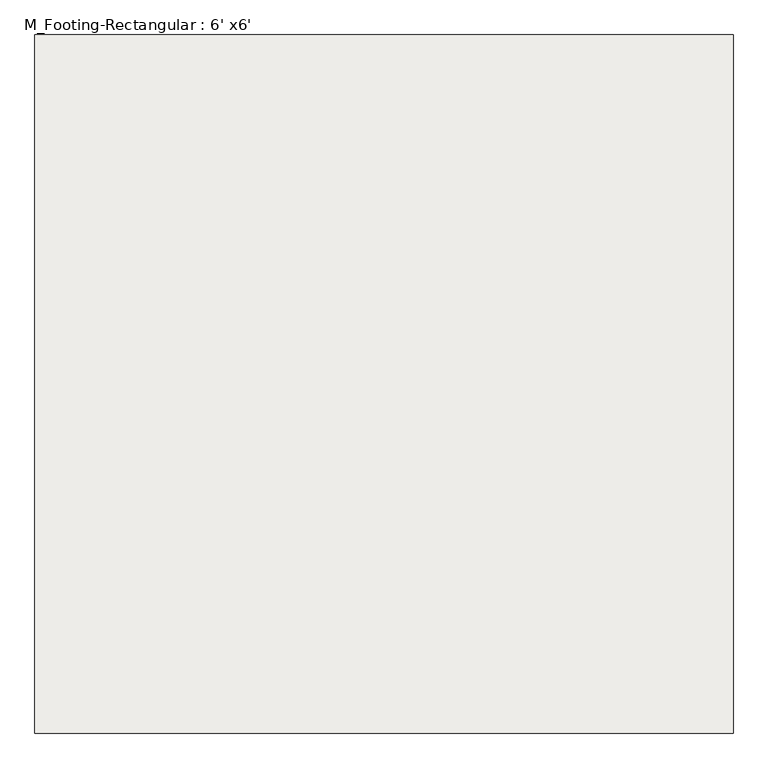
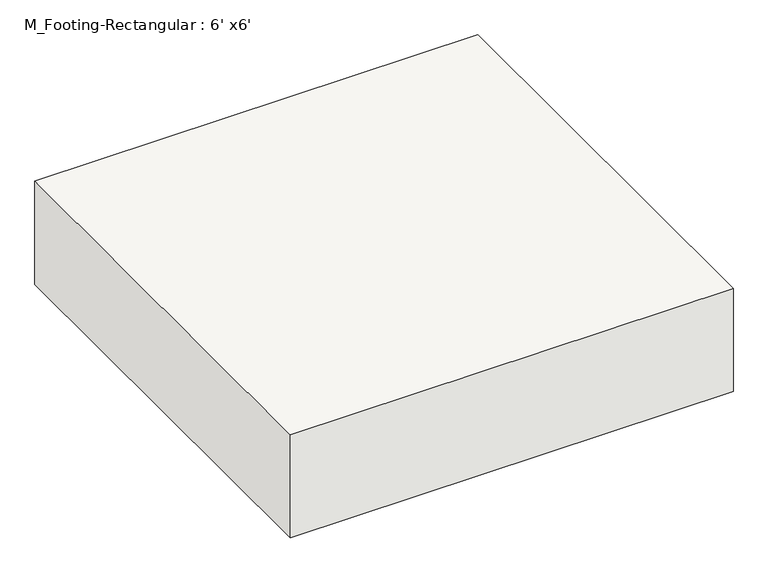
"""IFC4 building model written with IfcOpenShell, lengths in millimetres: slab geometry, M_Footing-Rectangular : 6' x6'."""

from ifc_helpers import new_model, si_unit, frame, origin, place, context, project, spatial, polyline, outline, extrude, source, transform, mapped, element, save


def m_footing_rectangular_6_x6_603268f9(model_context):
    return source(origin(), model_context, "Body", "SweptSolid", [
        extrude(outline(polyline([(914.4, 914.4), (914.4, -914.4), (-914.4, -914.4), (-914.4, 914.4), (914.4, 914.4)])), frame((0.0, 0.0, -450.0), z_axis=(0.0, 0.0, 1.0), x_axis=(1.0, 0.0, 0.0)), (0.0, 0.0, 1.0), 450.0),
    ])


if __name__ == "__main__":
    model = new_model("IFC4")
    model_context = context("Model", 3, world=origin())
    ifc_project = project(units=[si_unit("LENGTHUNIT", "METRE", prefix="MILLI")], contexts=[model_context])
    site = spatial("IfcSite", under=ifc_project)
    building = spatial("IfcBuilding", under=site)
    placement = place(None, origin())
    m_footing_rectangular_6_x6_shape = m_footing_rectangular_6_x6_603268f9(model_context)
    element("IfcSlab", 1, ObjectType="M_Footing-Rectangular : 6' x6'", at=placement, inside=building, context=model_context, shape_type="MappedRepresentation", body=[
        mapped(m_footing_rectangular_6_x6_shape, transform((0.0, 0.0, 0.0), x_axis=(1.0, 0.0, 0.0), y_axis=(0.0, 1.0, 0.0), z_axis=(0.0, 0.0, 1.0))),
    ])
    save(model, "model.ifc")

# Revit data of these elements
# Type "M_Footing-Rectangular : 6' x6'"
#   Width = 6' - 0"
#   Length = 6' - 0"
#   Foundation Thickness = 1' - 5.71654"
#   Structural Material [instance default] = Concrete, Cast-in-Place gray
#   Assembly Code = ""
# Element 1 (IfcSlab, "M_Footing-Rectangular : 6' x6'")
#   Materials on its faces: "Concrete, Cast-in-Place gray"
# Materials
#   "Concrete, Cast-in-Place gray": class "Concrete", colour RGB 192 192 192, transparency 0, Description = "Cast-in-place concrete", Cost = 0
